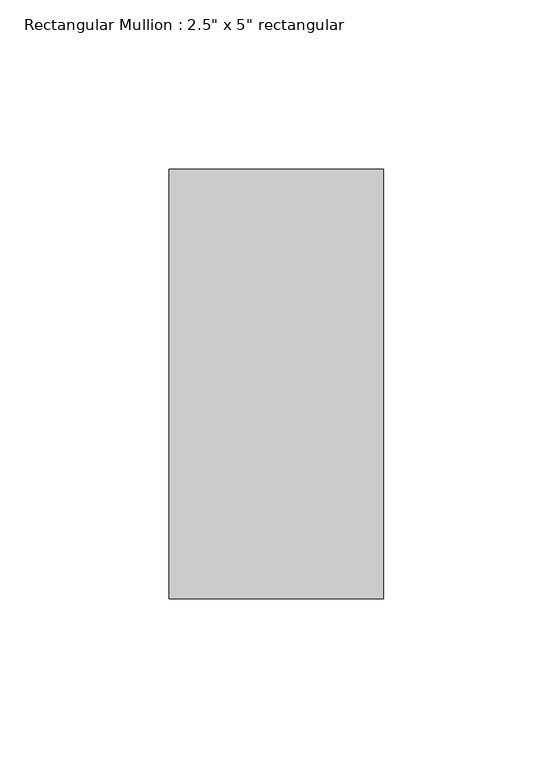
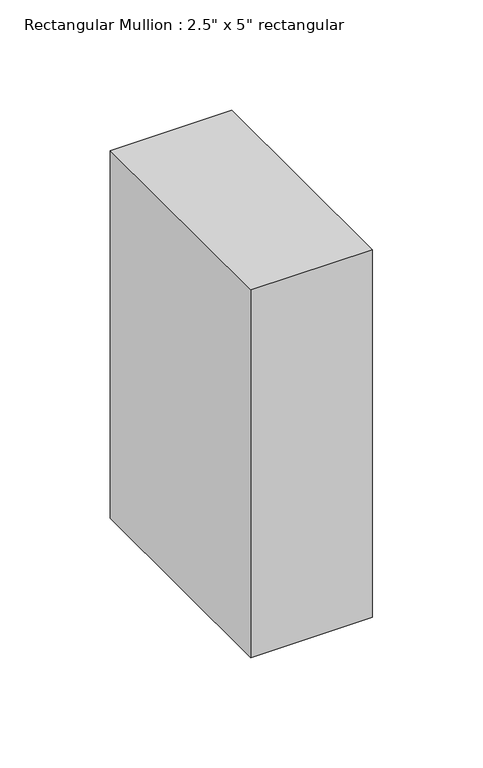
"""IFC4 building model written with IfcOpenShell, lengths in millimetres: member geometry."""

from ifc_helpers import new_model, si_unit, frame, origin, place, context, project, spatial, polyline, outline, extrude, source, transform, mapped, element, save


def member_a8054089(model_context):
    return source(origin(), model_context, "Body", "SweptSolid", [
        extrude(outline(polyline([(0.0, 63.5), (0.0, -63.5), (-63.5, -63.5), (-63.5, 63.5), (0.0, 63.5)])), frame((0.0, 0.0, -203.2), z_axis=(0.0, 0.0, 1.0), x_axis=(1.0, 0.0, 0.0)), (0.0, 0.0, 1.0), 203.2),
    ])


if __name__ == "__main__":
    model = new_model("IFC4")
    model_context = context("Model", 3, world=origin())
    ifc_project = project(units=[si_unit("LENGTHUNIT", "METRE", prefix="MILLI")], contexts=[model_context])
    site = spatial("IfcSite", under=ifc_project)
    building = spatial("IfcBuilding", under=site)
    placement = place(None, origin())
    member_shape = member_a8054089(model_context)
    element("IfcMember", 1, ObjectType="Rectangular Mullion : 2.5\" x 5\" rectangular", at=placement, inside=building, context=model_context, shape_type="MappedRepresentation", body=[
        mapped(member_shape, transform((0.0, 0.0, 0.0), x_axis=(1.0, 0.0, 0.0), y_axis=(0.0, 1.0, 0.0), z_axis=(0.0, 0.0, 1.0))),
    ])
    save(model, "model.ifc")

# Revit data of these elements
# Type "Rectangular Mullion : 2.5\" x 5\" rectangular"
#   built-in parameter 1007304 = 0.416667 (stored number, unit not read)
#   built-in parameter 1007301 = 0.104167 (stored number, unit not read)
#   built-in parameter 1007300 = 0.104167 (stored number, unit not read)
# Element 1 (IfcMember, "Rectangular Mullion : 2.5\" x 5\" rectangular")
#   Materials on its faces: "Aluminum"
# Materials
#   "Aluminum": class "Metal", colour RGB 247 247 247, transparency 0, Description = "Aluminum 6061", Cost = 0
